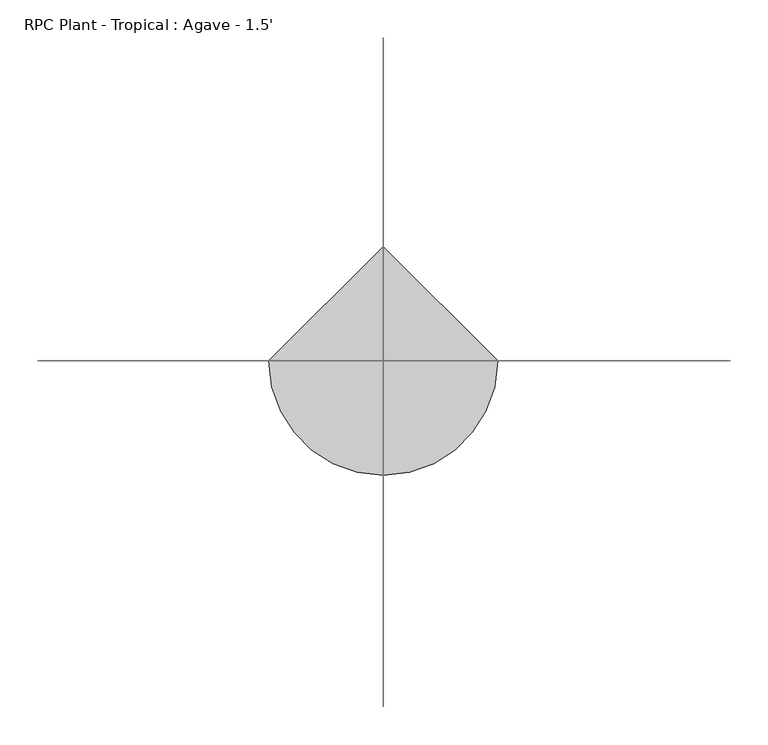
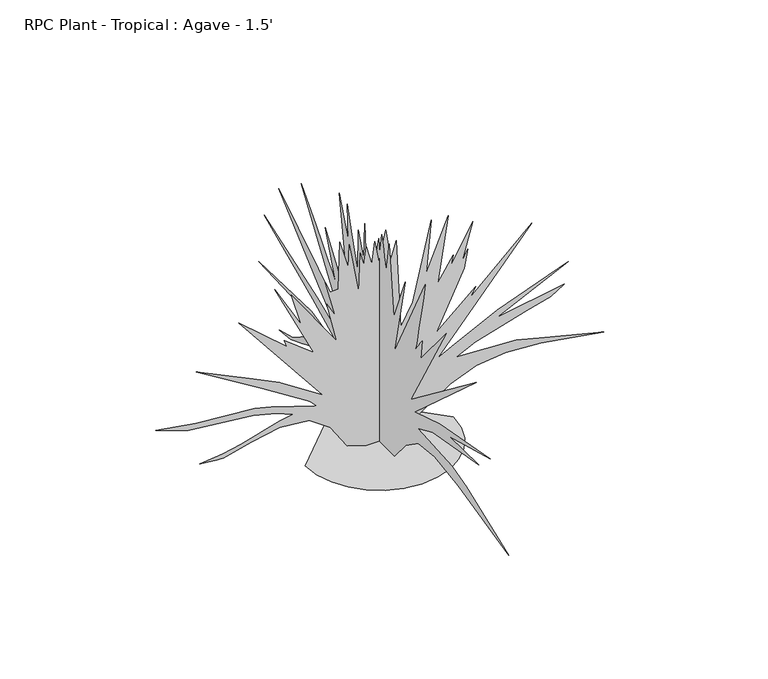
"""IFC4 building model written with IfcOpenShell, lengths in millimetres: geographic element geometry, RPC Plant - Tropical : Agave - 1.5'."""

from ifc_helpers import new_model, si_unit, origin, place, context, project, spatial, triangles, source, transform, mapped, element, save


def rpc_plant_tropical_agave_1_5_93a2a214(model_context):
    return source(origin(), model_context, "Body", "Tessellation", [
        triangles([(-150.7087333, 0.0, 9.4e-06), (-146.7244834, -34.5323444, 9.4e-06), (-135.3772836, -66.2450299, 9.4e-06), (-117.5759356, -94.2289958, 9.4e-06), (-94.2289958, -117.5759356, 9.4e-06), (-66.2450299, -135.3772836, 9.4e-06), (-34.5323444, -146.7244834, 9.4e-06), (6.6e-06, -150.7087333, 9.4e-06), (34.5323444, -146.7244834, 9.4e-06), (66.2450299, -135.3772836, 9.4e-06), (94.2289958, -117.5759356, 9.4e-06), (117.5759356, -94.2289958, 9.4e-06), (135.3772836, -66.2450299, 9.4e-06), (146.7244834, -34.5323444, 9.4e-06), (150.7087333, 1.32e-05, 9.4e-06), (-1.98e-05, 150.7087333, 9.4e-06), (-24.9398476, 1.1e-06, 2.5e-06), (-65.4258802, 2.1e-06, 13.141818), (-99.6620581, 5e-07, 65.0964399), (-143.0435126, 6e-07, 95.6658721), (-202.3246234, 2.8e-06, 101.1403381), (-259.7355268, 6e-06, 89.1792132), (-316.7763402, 9.4e-06, 74.9889865), (-329.6211594, 9.9e-06, 75.5035945), (-365.3285002, 1.12e-05, 79.1975187), (-318.313056, 8.9e-06, 84.1103911), (-282.3389982, 6.9e-06, 91.7898278), (-203.1008479, 2e-06, 114.8573697), (-175.7107319, 5e-07, 119.829677), (-208.3624635, 1.2e-06, 133.0887423), (-256.7688111, 2.5e-06, 145.787731), (-389.2832517, 7.5e-06, 160.0767662), (-455.2115313, 9e-06, 182.6248811), (-373.9467241, 6.3e-06, 169.0808314), (-253.2813787, 1.6e-06, 159.2306877), (-220.3573709, 6e-07, 151.0805947), (-127.6907252, -1.6e-06, 121.0610699), (-140.4735387, -1.9e-06, 135.3043865), (-238.3492232, -1.3e-06, 197.06021), (-372.7148226, -4e-07, 279.8955245), (-256.342093, -2.1e-06, 224.048243), (-204.0302424, -2.9e-06, 198.6317166), (-115.3780683, -3.3e-06, 140.7615752), (-286.5249345, -8.6e-06, 355.0033673), (-188.0233888, -7.9e-06, 270.045399), (-192.9487059, -8.5e-06, 284.8205873), (-133.8471808, -8.3e-06, 238.0324729), (-212.6492294, -1.47e-05, 401.7927715), (-158.472758, -1.14e-05, 306.9846414), (-179.4046562, -1.47e-05, 378.3993593), (-87.0585669, -1.09e-05, 246.6514781), (-106.7590813, -1.52e-05, 332.8418567), (-89.5210982, -1.41e-05, 302.0595786), (-110.4530055, -1.79e-05, 380.860619), (-99.717687, -1.69e-05, 356.9287222), (-83.2732056, -1.76e-05, 356.9490335), (-80.9021112, -2.37e-05, 457.2003633), (-63.426897, -2.09e-05, 396.9718449), (-61.2016014, -2.38e-05, 444.8864347), (-41.5013458, -1.82e-05, 335.3031163), (-39.0385601, -2.33e-05, 419.0317629), (-31.650966, -2.19e-05, 390.7107445), (-26.7259009, -2.44e-05, 428.8818884), (-15.6443803, -2.24e-05, 387.0175833), (-9.4879996, -2.54e-05, 433.8069511), (-0.8690236, -2.3e-05, 387.0175833), (12.6750416, -2.74e-05, 451.043399), (23.7565623, -2.39e-05, 383.3244221), (34.8381601, -2.66e-05, 420.261121), (43.4571494, -1.56e-05, 230.6448788), (68.0824677, -1.94e-05, 276.2023633), (105.4982208, -3.08e-05, 439.9537416), (95.1708261, -2.38e-05, 329.146152), (140.4829403, -3.22e-05, 436.9539974), (118.5650104, -2.3e-05, 299.5957755), (150.578436, -2.74e-05, 348.8489465), (145.6533642, -2.58e-05, 326.6848924), (189.9794467, -3.25e-05, 406.7178343), (167.81641, -2.69e-05, 327.9167939), (180.1290669, -2.88e-05, 351.3102061), (173.4681726, -2.62e-05, 313.009528), (116.102479, -1.66e-05, 193.7063995), (196.1359024, -2.44e-05, 265.1203362), (183.8229911, -2.26e-05, 244.1889286), (310.6447741, -3.51e-05, 361.1603316), (118.5650104, -1.34e-05, 138.2987895), (158.4747927, -1.63e-05, 158.0775423), (240.4617396, -2.24e-05, 198.6317166), (384.5207517, -3.19e-05, 252.8079337), (239.2306011, -2.13e-05, 182.6248811), (376.7864491, -2.88e-05, 206.3655105), (349.174072, -2.66e-05, 189.8819236), (300.4111145, -2.36e-05, 176.0696308), (195.4584909, -1.73e-05, 146.0828801), (156.7348917, -1.44e-05, 127.2172711), (278.6305944, -1.94e-05, 121.0610699), (336.3953462, -2.1e-05, 106.1004551), (457.1673348, -2.45e-05, 75.5035945), (329.0750444, -2.01e-05, 96.2046111), (257.431743, -1.73e-05, 101.1027496), (197.4574787, -1.42e-05, 94.105802), (144.7537007, -1.07e-05, 73.3684686), (86.5066293, -5.8e-06, 34.1325482), (33.0588878, -1.4e-06, 0.0), (9e-07, 20.0836192, 9.1e-06), (2.1e-06, 47.8000438, 9.9e-06), (3.7e-06, 68.4088604, 20.0829062), (6.2e-06, 99.6950775, 59.1195655), (8.3e-06, 132.7178983, 80.7177112), (1.03e-05, 174.2748821, 84.8467378), (1.15e-05, 208.5839434, 72.8693576), (1.35e-05, 272.2425033, 45.8366235), (1.48e-05, 311.9833551, 30.2844433), (1.65e-05, 353.3269798, 25.0212039), (1.48e-05, 305.3793614, 38.860505), (1.34e-05, 249.7515432, 74.8251566), (1.18e-05, 199.8564965, 97.660536), (1.01e-05, 161.2479701, 96.4354927), (1.17e-05, 188.527337, 110.366392), (1.51e-05, 256.1160167, 122.0234748), (2.29e-05, 425.717038, 129.5510222), (1.47e-05, 238.8183625, 134.6051196), (1.09e-05, 164.9452008, 118.743824), (8.2e-06, 119.3844099, 96.4354927), (1.1e-05, 159.9457058, 127.6671074), (1.54e-05, 233.8196305, 165.2718342), (2.53e-05, 406.273312, 240.4952587), (1.5e-05, 217.8867004, 177.6998184), (1.1e-05, 147.7036569, 148.1491784), (2.57e-05, 354.5588814, 329.146152), (1.25e-05, 146.2032761, 198.5547591), (2.38e-05, 274.5259576, 388.2494848), (2.18e-05, 248.7817623, 359.4966614), (1.99e-05, 223.9913424, 331.6328098), (1.81e-05, 201.1074557, 305.5495545), (1.65e-05, 181.0833509, 282.1358129), (1.52e-05, 164.872549, 262.2780679), (1.42e-05, 153.4283166, 246.8711776), (1.37e-05, 147.7036569, 236.8013344), (1.88e-05, 190.798601, 345.1532418), (1.51e-05, 148.9134577, 283.7461616), (1.48e-05, 144.9251474, 278.3410409), (1.44e-05, 140.1001603, 272.7403471), (1.4e-05, 134.5776867, 266.9770725), (1.35e-05, 128.4971803, 261.086807), (1.31e-05, 121.9980766, 255.0974924), (1.26e-05, 115.2200837, 249.0439011), (1.21e-05, 108.3028915, 242.95779), (1.97e-05, 140.3160628, 449.8114975), (1.58e-05, 109.53403, 367.3172959), (1.82e-05, 113.2279542, 442.4251751), (1.61e-05, 98.452766, 393.1745476), (1.29e-05, 75.0583319, 320.5279281), (1.55e-05, 73.826939, 410.4109955), (1.32e-05, 55.357822, 358.699072), (1.53e-05, 51.6638932, 437.5001123), (1.36e-05, 47.2595336, 384.1829453), (1.1e-05, 27.0383205, 327.9167939), (1.31e-05, 1.1814591, 436.2682108), (1.2e-05, -1.2811313, 405.4859327), (1.3e-05, -8.5500533, 450.4566616), (1.25e-05, -11.9783704, 436.1437634), (1.19e-05, -15.2441015, 422.2677209), (1.14e-05, -18.1847128, 409.2629188), (1.09e-05, -20.6375916, 397.5687561), (1.05e-05, -22.4401819, 387.6195451), (1.03e-05, -23.4298925, 379.852214), (1.01e-05, -23.4441676, 374.7036547), (1.18e-05, -34.5257405, 446.1183363), (6.6e-06, -50.5323262, 298.3664174), (7.8e-06, -92.3958773, 399.3315119), (4.4e-06, -52.9948575, 225.7198161), (5.7e-06, -162.5786665, 436.2682108), (5.1e-06, -155.9520543, 404.0000133), (4.4e-06, -149.5159464, 372.9078704), (3.8e-06, -143.4613468, 344.1651844), (3.3e-06, -137.9787509, 318.9480463), (2.9e-06, -133.2591716, 298.4324563), (2.7e-06, -129.4933677, 283.7918891), (2.6e-06, -126.87158, 276.2023633), (2.5e-06, -126.0089964, 274.2135312), (2.5e-06, -127.1682462, 275.2524031), (2.5e-06, -130.0120315, 278.8160301), (2.5e-06, -134.204054, 284.398956), (2.5e-06, -139.4067433, 291.4957067), (2.4e-06, -145.2835467, 299.6034059), (2.4e-06, -151.4971481, 308.2165429), (1.4e-06, -145.3409469, 266.3522378), (6e-07, -236.4556433, 375.9355562), (-2e-07, -110.8649898, 157.9992949), (-5.3e-06, -341.1146439, 334.0712148), (-1.4e-06, -124.4090487, 138.2990438), (-4.6e-06, -213.0612137, 166.6183), (-1.15e-05, -391.2898516, 199.4396978), (-6.2e-06, -246.3057688, 160.4618262), (-1.09e-05, -351.4651749, 162.9246119), (-4.5e-06, -189.3266705, 133.5012353), (-2.8e-06, -135.490567, 109.9795515), (-8.4e-06, -257.3885589, 102.5916939), (-1.11e-05, -306.6392046, 89.0476442), (-1.94e-05, -455.623025, 31.1775097), (-1.03e-05, -278.0057598, 72.8693576), (-6.2e-06, -195.1343828, 85.0082832), (-3.8e-06, -137.6096873, 78.9734862), (-2.8e-06, -94.1832773, 48.8668437), (-2.4e-06, -52.6021717, 6.9e-06), (-9e-07, -19.1255291, 7.9e-06)], [[15, 16, 1], [14, 15, 1], [14, 1, 2], [13, 14, 2], [13, 2, 3], [13, 3, 4], [12, 13, 4], [11, 12, 4], [11, 4, 5], [11, 5, 6], [11, 6, 7], [11, 7, 8], [11, 8, 9], [11, 9, 10], [47, 48, 49], [97, 98, 99], [88, 89, 90], [39, 40, 41], [84, 85, 86], [71, 72, 73], [53, 54, 55], [32, 33, 34], [43, 44, 45], [24, 25, 26], [58, 59, 60], [77, 78, 79], [73, 74, 75], [60, 61, 62], [51, 52, 53], [56, 57, 58], [82, 83, 84], [79, 80, 81], [64, 65, 66], [49, 50, 51], [68, 69, 70], [75, 76, 77], [90, 91, 92], [90, 92, 93], [66, 67, 68], [82, 84, 86], [90, 93, 94], [62, 63, 64], [47, 49, 51], [39, 41, 42], [45, 46, 47], [43, 45, 47], [38, 39, 42], [38, 42, 43], [31, 32, 34], [31, 34, 35], [23, 24, 26], [56, 58, 60], [87, 88, 90], [87, 90, 94], [87, 94, 95], [37, 38, 43], [86, 87, 95], [71, 73, 75], [96, 97, 99], [96, 99, 100], [95, 96, 100], [95, 100, 101], [95, 101, 102], [53, 55, 56], [53, 56, 60], [22, 23, 26], [22, 26, 27], [22, 27, 28], [21, 22, 28], [60, 62, 64], [43, 47, 51], [30, 31, 35], [30, 35, 36], [30, 36, 37], [29, 30, 37], [86, 95, 102], [21, 28, 29], [20, 21, 29], [20, 29, 37], [19, 20, 37], [86, 102, 103], [66, 68, 70], [64, 66, 70], [60, 64, 70], [53, 60, 70], [51, 53, 70], [43, 51, 70], [77, 79, 81], [77, 81, 82], [75, 77, 82], [71, 75, 82], [70, 71, 82], [70, 82, 86], [43, 70, 86], [43, 86, 103], [43, 103, 104], [43, 104, 17], [43, 17, 18], [43, 18, 19], [43, 19, 37], [120, 121, 122], [193, 194, 195], [190, 191, 192], [126, 127, 128], [155, 156, 157], [131, 132, 133], [200, 201, 202], [113, 114, 115], [195, 196, 197], [129, 130, 131], [131, 133, 134], [170, 171, 172], [188, 189, 190], [131, 134, 135], [148, 149, 150], [139, 140, 141], [131, 135, 136], [150, 151, 152], [168, 169, 170], [172, 173, 174], [131, 136, 137], [158, 159, 160], [172, 174, 175], [131, 137, 138], [153, 154, 155], [131, 138, 139], [172, 175, 176], [160, 161, 162], [172, 176, 177], [186, 187, 188], [172, 177, 178], [112, 113, 115], [112, 115, 116], [111, 112, 116], [111, 116, 117], [160, 162, 163], [172, 178, 179], [172, 179, 180], [172, 180, 181], [139, 141, 142], [193, 195, 197], [185, 186, 188], [192, 193, 197], [192, 197, 198], [155, 157, 158], [150, 152, 153], [148, 150, 153], [139, 142, 143], [199, 200, 202], [119, 120, 122], [119, 122, 123], [118, 119, 123], [199, 202, 203], [198, 199, 203], [198, 203, 204], [184, 185, 188], [110, 111, 117], [110, 117, 118], [109, 110, 118], [160, 163, 164], [118, 123, 124], [109, 118, 124], [139, 143, 144], [125, 126, 128], [125, 128, 129], [183, 184, 188], [139, 144, 145], [153, 155, 158], [108, 109, 124], [139, 145, 146], [160, 164, 165], [158, 160, 165], [158, 165, 166], [158, 166, 167], [158, 167, 168], [158, 168, 170], [182, 183, 188], [124, 125, 129], [182, 188, 190], [181, 182, 190], [172, 181, 190], [139, 146, 147], [131, 139, 147], [131, 147, 148], [158, 170, 172], [153, 158, 172], [148, 153, 172], [198, 204, 205], [131, 148, 172], [129, 131, 172], [124, 129, 172], [124, 172, 190], [108, 124, 190], [107, 108, 190], [106, 107, 190], [105, 106, 190], [207, 105, 190], [206, 207, 190], [205, 206, 190], [198, 205, 190], [192, 198, 190]], closed=False),
    ])


if __name__ == "__main__":
    model = new_model("IFC4")
    model_context = context("Model", 3, world=origin())
    ifc_project = project(units=[si_unit("LENGTHUNIT", "METRE", prefix="MILLI")], contexts=[model_context])
    site = spatial("IfcSite", under=ifc_project)
    building = spatial("IfcBuilding", under=site)
    placement = place(None, origin())
    rpc_plant_tropical_agave_1_5_shape = rpc_plant_tropical_agave_1_5_93a2a214(model_context)
    element("IfcGeographicElement", 1, ObjectType="RPC Plant - Tropical : Agave - 1.5'", at=placement, inside=building, context=model_context, shape_type="MappedRepresentation", body=[
        mapped(rpc_plant_tropical_agave_1_5_shape, transform((0.0, 0.0, 0.0), x_axis=(1.0, 0.0, 0.0), y_axis=(0.0, 1.0, 0.0), z_axis=(0.0, 0.0, 1.0))),
    ])
    save(model, "model.ifc")

# Revit data of these elements
# Type "RPC Plant - Tropical : Agave - 1.5'"
#   built-in parameter 1005198 = "{2, 15},{39, RPC-16-G1GJ-63FX-7K5P-N000-ST1L-LVER-AU},{1, 0},{1, 0},{2, 35},{1, 8},{5, Color},{1, 0},{1, 0},{3, 0.8},{3, 0.8},{3, 0.8},{1, 8},{7, BBoxMin},{1, 0},{1, 0},{1, 0},{1, 0},{1, 0},{1, 8},{7, BBoxMax},{1, 0},{1, 0},{1, 0},{1, 0},{1, 0},{2, 11},{9, RPCTypeId},{1, 0},{1, 0},{39, RPC-16-G1GJ-63FX-7K5P-N000-ST1L-LVER-AU},{1, 6},{14, RPCPlantHeight},{1, 0},{1, 0},{3, 1.5},{2, 11},{7, keyword},{1, 0},{1, 0},{88, :Geometry:RPC:Agave:agave:agave americana marginata:mesqual:south western:tropical:plant},{2, 11},{8, category},{1, 0},{1, 0},{17, :Plants [General]},{2, 11},{12, LocalizedUID},{1, 0},{1, 0},{5, Agave},{2, 14},{6, Height},{1, 0},{1, 0},{3, 1.5},{1, 2},{16, Cast Reflections},{1, 0},{1, 0},{1, 0},{1, 2},{12, Cast Shadows},{1, 0},{1, 0},{1, 1},{1, 2},{9, Lock View},{1, 0},{1, 0},{1, 0},{1, 4},{5, ViewC},{1, 0},{1, 0},{1, 0},{2, 11},{20, AdvancedUIDefinition},{1, 0},{1, 0},{0, },{2, 11},{10, AssetLibID},{1, 0},{1, 0},{36, 4D3F6E72-3F99-4203-98E9-AF80B3C7A7A4},{2, 11},{10, BaseSchema},{1, 0},{1, 0},{9, RPCSchema},{2, 11},{12, ExchangeGUID},{1, 0},{1, 0},{0, },{1, 2},{6, Hidden},{1, 0},{1, 0},{1, 0},{1, 4},{11, RPCCategory},{1, 0},{1, 0},{1, 0},{2, 11},{8, RPCImage},{1, 0},{1, 0},{0, },{1, 4},{13, SchemaVersion},{1, 0},{1, 0},{1, 4},{2, 11},{12, UIDefinition},{1, 0},{1, 0},{0, },{2, 11},{6, UIName},{1, 0},{1, 0},{39, RPC-16-G1GJ-63FX-7K5P-N000-ST1L-LVER-AU},{2, 11},{11, VersionGUID},{1, 0},{1, 0},{9, RPCSchema},{2, 11},{9, assettype},{1, 0},{1, 0},{11, RPCGeometry},{2, 11},{11, description},{1, 0},{1, 0},{0, },{2, 11},{9, localname},{1, 0},{1, 0},{3, RPC},{2, 11},{9, localtype},{1, 0},{1, 0},{3, RPC},{1, 4},{8, revision},{1, 0},{1, 0},{1, 1},{2, 11},{9, thumbnail},{1, 0},{1, 0},{0, },{1, 4},{7, version},{1, 0},{1, 0},{1, 1},{1, 2},{20, RPC_Cast Reflections},{1, 0},{1, 0},{1, 1},{1, 2},{16, RPC_Cast Shadows},{1, 0},{1, 0},{1, 1},{1, 2},{13, RPC_Lock View},{1, 0},{1, 0},{1, 0},{1, 4},{9, RPC_ViewC},{1, 0},{1, 0},{1, 0},{21, assetlibrary_base.fbx},{1, 5},"
#   built-in parameter 1005195 = "RPC-16-G1GJ-63FX-7K5P-N000-ST1L-LVER-AU"
#   Type Comments = "Agave"
#   Assembly Code = "G2050500"
#   Height = 1' - 6"
#   Default Elevation = 0
